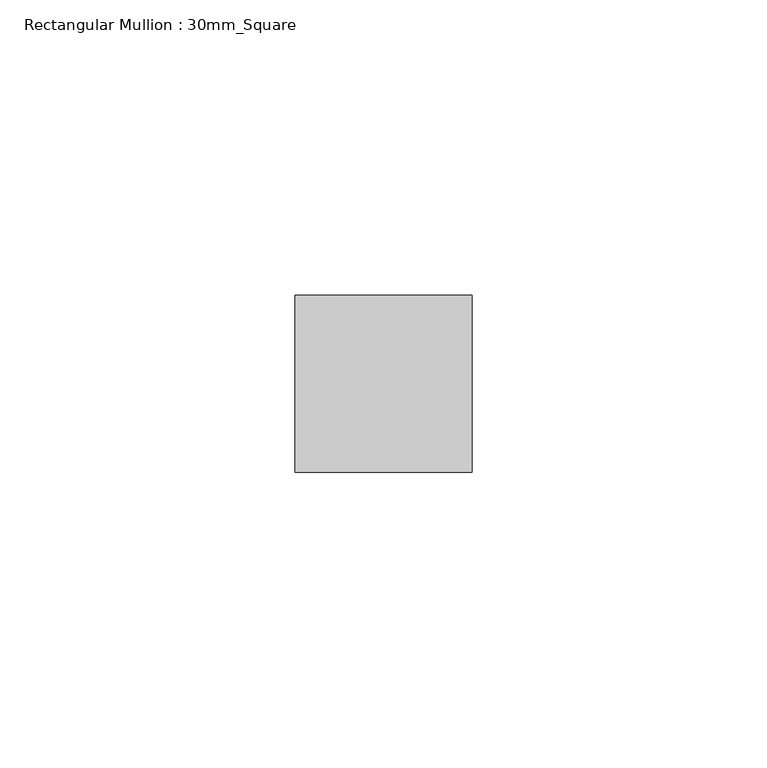
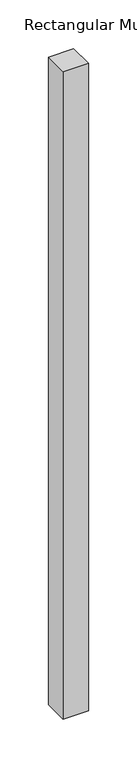
"""IFC4 building model written with IfcOpenShell, lengths in millimetres: member geometry, Rectangular Mullion : 30mm_Square."""

from ifc_helpers import new_model, si_unit, frame, origin, place, context, project, spatial, polyline, outline, extrude, source, transform, mapped, element, save


def rectangular_mullion_30mm_square_fdabec93(model_context):
    return source(origin(), model_context, "Body", "SweptSolid", [
        extrude(outline(polyline([(15.0, 15.0), (15.0, -15.0), (-15.0, -15.0), (-15.0, 15.0), (15.0, 15.0)])), frame((0.0, 0.0, -812.9157956), z_axis=(0.0, 0.0, 1.0), x_axis=(1.0, 0.0, 0.0)), (0.0, 0.0, 1.0), 812.9157956),
    ])


if __name__ == "__main__":
    model = new_model("IFC4")
    model_context = context("Model", 3, world=origin())
    ifc_project = project(units=[si_unit("LENGTHUNIT", "METRE", prefix="MILLI")], contexts=[model_context])
    site = spatial("IfcSite", under=ifc_project)
    building = spatial("IfcBuilding", under=site)
    placement = place(None, origin())
    rectangular_mullion_30mm_square_shape = rectangular_mullion_30mm_square_fdabec93(model_context)
    element("IfcMember", 1, ObjectType="Rectangular Mullion : 30mm_Square", at=placement, inside=building, context=model_context, shape_type="MappedRepresentation", body=[
        mapped(rectangular_mullion_30mm_square_shape, transform((0.0, 0.0, 0.0), x_axis=(1.0, 0.0, 0.0), y_axis=(0.0, 1.0, 0.0), z_axis=(0.0, 0.0, 1.0))),
    ])
    save(model, "model.ifc")

# Revit data of these elements
# Type "Rectangular Mullion : 30mm_Square"
#   Keynote = "H11"
#   built-in parameter 1007304 = 0.0984252 (stored number, unit not read)
#   built-in parameter 1007301 = 0.0492126 (stored number, unit not read)
#   built-in parameter 1007300 = 0.0492126 (stored number, unit not read)
# Element 1 (IfcMember, "Rectangular Mullion : 30mm_Square")
#   Materials on its faces: "Aluminium"
# Materials
#   "Aluminium": class "Metal", colour RGB 247 247 247, transparency 0, Description = "Aluminium 6061", Cost = 0
